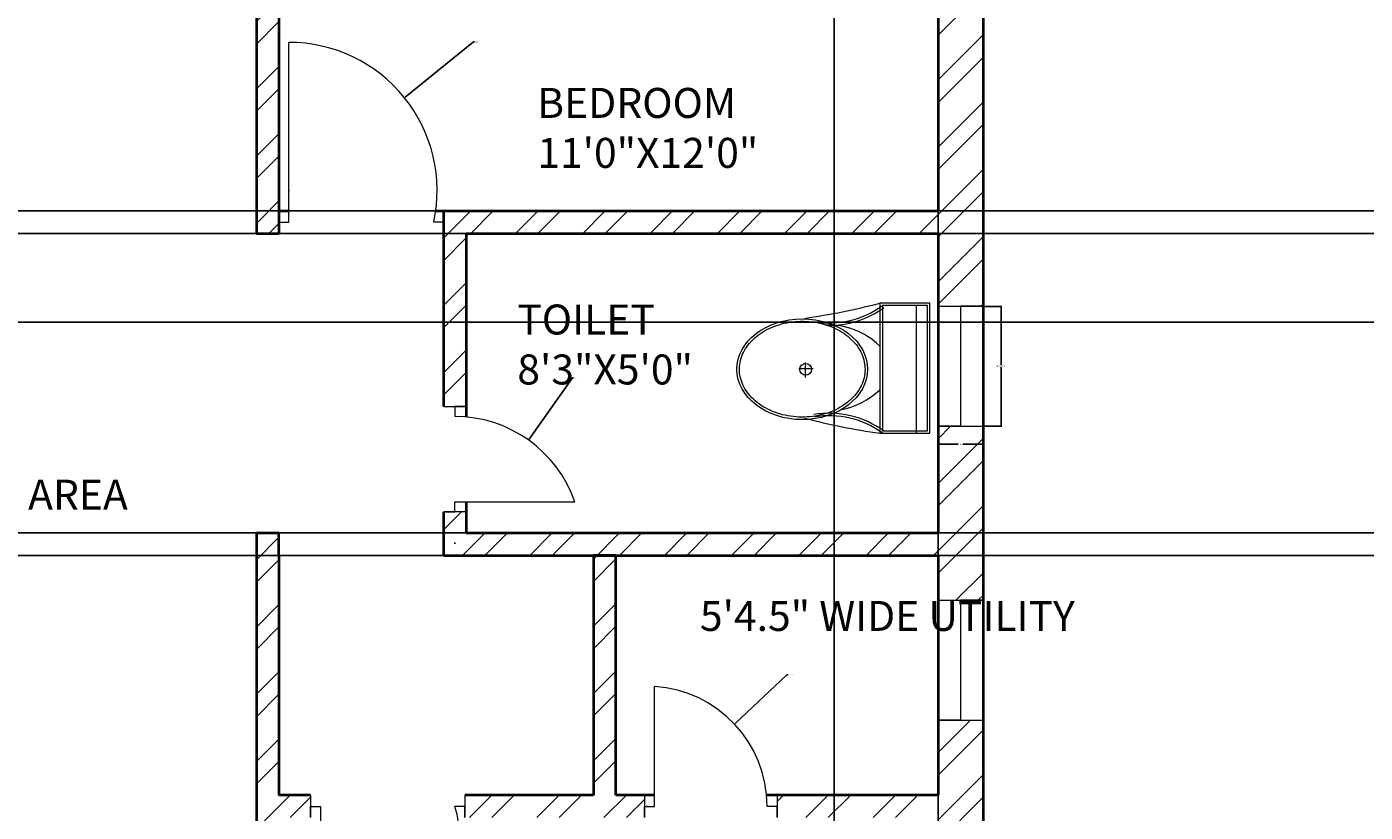
# Model space of a CAD drawing. Units: inches. Extents: x 1355 to 2746, y 1171 to 2751.
# Tile 12 of 24: x 1749 to 2017, y 1866 to 2023. Entities that reach past the tile are written whole.
import ezdxf

# ---------------------------------------------------------------- set-up
doc = ezdxf.new("R2010")
doc.units = ezdxf.units.IN
for name, color, linetype, lineweight in [('A-ANNO-DIMS', 2, 'Continuous', 18), ('A-AREA-IDEN', 7, 'Continuous', 18), ('A-DOOR', 3, 'Continuous', 20), ('A-FLOR-FIXT', 9, 'Continuous', 18), ('A-GLAZ', 4, 'Continuous', 18), ('A-WALL', 7, 'Continuous', 40), ('A-WALL-PATT', 252, 'Continuous', 13)]:
    doc.layers.add(name, color=color, linetype=linetype, lineweight=lineweight)
doc.styles.get("Standard").update_dxf_attribs({"font": 'arial.ttf'})
doc.dimstyles.get("Standard").update_dxf_attribs({"dimtxt": 0.18, "dimasz": 0.18, "dimexe": 0.18, "dimexo": 0.0625, "dimgap": 0.09, "dimtad": 0, "dimtih": 1, "dimtoh": 1, "dimdec": 4, "dimzin": 0, "dimdsep": 46, "dimtxsty": 'Standard', "dimcen": 0.09, "dimadec": 0, "dimazin": 0, "dimtfac": 1, "dimtdec": 4, "dimtofl": 0, "dimtmove": 0, "dimatfit": 3, "dimfxl": 1, "dimtolj": 1, "dimtzin": 0, "dimarcsym": 0})

# ---------------------------------------------------------------- blocks, each defined once
blk = doc.blocks.new('A$C31115884')
for p, q in [((283.1, 497.7), (223.4, 497.7)), ((257.5, 466.4), (257.5, 523.2)), ((0, 200), (0, 0)), ((520, 200), (0, 200)), ((10, 190), (10, 10)), ((510, 190), (10, 190)), ((510, 10), (510, 190)), ((520, 0), (520, 200)), ((510, 54.5), (0, 54.5)), ((10, 10), (510, 10)), ((0, 0), (520, 0))]:
    blk.add_line(p, q)
blk.add_circle((255.6, 496.4), 23.6)
for centre, radius, start, end in [((2777.7, -204.6), 2807, 165.4549, 171.7133), ((3237, 905), 2807, 188.2867, 194.5451), ((-294.5, 403.3), 364.7, 324.2091, 9.3499), ((-294.5, 403.3), 374.7, 324.2091, 9.3499), ((805.8, 403.3), 364.7, 170.6501, 215.7909), ((139.5, 406.2), 293.5, 315.8436, 2.6563), ((805.8, 403.3), 374.7, 179.2036, 215.7909), ((383.6, 406.2), 293.5, 190.2774, 224.1564)]:
    blk.add_arc(centre, radius, start, end)
blk.add_ellipse((256.2, 509.9), major_axis=(0, -260.7), ratio=0.772727)
blk.add_open_spline([(256.2, 259.2), (263.1, 259.2), (270, 259.7), (287.8, 262.3), (298.7, 265.1), (319.9, 273.1), (330.2, 278.4), (350.1, 291.1), (359.7, 298.7), (377.7, 315.9), (386.2, 325.5), (401.7, 346.6), (408.8, 358.1), (421.3, 382.5), (426.8, 395.5), (435.9, 422.4), (439.5, 436.4), (444.8, 465.1), (446.5, 479.7), (447.9, 509.2), (447.6, 524), (445, 553.3), (442.7, 567.8), (436.3, 596), (432.1, 609.7), (421.9, 636), (416, 648.6), (402.5, 672.1), (395, 683), (378.6, 703), (369.8, 712.1), (351.1, 728), (341.3, 734.8), (320.9, 746.2), (310.4, 750.7), (288.9, 757.3), (278, 759.4), (256, 761), (245, 760.6), (223.1, 757.2), (212.3, 754.3), (191.1, 746.1), (180.8, 740.7), (160.9, 727.8), (151.4, 720.1), (133.5, 702.7), (125.1, 693), (109.6, 671.7), (102.6, 660.2), (90.2, 635.7), (84.9, 622.7), (76, 595.6), (72.4, 581.6), (67.2, 552.9), (65.6, 538.2), (64.4, 508.8), (64.8, 494), (67.5, 464.7), (69.9, 450.2), (76.6, 422), (80.8, 408.3), (91.1, 382.2), (97.2, 369.7), (110.8, 346.3), (118.4, 335.4), (134.8, 315.6), (143.7, 306.7), (162.4, 290.9), (172.3, 284.2), (192.8, 273), (203.3, 268.6), (224.8, 262.2), (235.8, 260.2), (249.9, 259.3), (253, 259.2), (256.2, 259.2)], degree=3, knots=[0, 0, 0, 0, 0.110105, 0.110105, 0.285049, 0.285049, 0.459994, 0.459994, 0.634938, 0.634938, 0.809882, 0.809882, 0.984827, 0.984827, 1.159771, 1.159771, 1.334715, 1.334715, 1.50966, 1.50966, 1.684604, 1.684604, 1.859549, 1.859549, 2.034493, 2.034493, 2.209437, 2.209437, 2.384382, 2.384382, 2.559326, 2.559326, 2.73427, 2.73427, 2.909215, 2.909215, 3.084159, 3.084159, 3.259103, 3.259103, 3.434048, 3.434048, 3.608992, 3.608992, 3.783936, 3.783936, 3.958881, 3.958881, 4.133825, 4.133825, 4.30877, 4.30877, 4.483714, 4.483714, 4.658658, 4.658658, 4.833603, 4.833603, 5.008547, 5.008547, 5.183491, 5.183491, 5.358436, 5.358436, 5.53338, 5.53338, 5.708324, 5.708324, 5.883269, 5.883269, 6.058213, 6.058213, 6.233158, 6.233158, 6.283185, 6.283185, 6.283185, 6.283185])
blk = doc.blocks.new('WINDOW-PLAN-24')
for p, q in [((0, 24), (9, 24)), ((9, 24), (4.5, 24)), ((4.5, 24), (4.5, 0)), ((4.5, 0), (0, 0)), ((0, 0), (9, 0))]:
    blk.add_line(p, q)
blk = doc.blocks.new('WINDOW-PLAN-24-2')
for p, q in [((0, 24), (9, 24)), ((9, 24), (4.5, 24)), ((4.5, 24), (4.5, 0)), ((4.5, 0), (0, 0)), ((0, 0), (0, 0)), ((0, 0), (9, 0))]:
    blk.add_line(p, q)
blk = doc.blocks.new('DOOR-UTILITY-N')
for p, q in [((2, 2.25), (2, 26.25)), ((0, 4.5), (0, 0)), ((26.56, 4.5), (26.56, 0)), ((0, 0), (0, 2.25)), ((0, 2.25), (2, 2.25)), ((26.56, 2.25), (24.56, 2.25)), ((26.56, 0), (26.56, 2.25))]:
    blk.add_line(p, q)
blk.add_arc((0.51, 2.25), 24.05, 0, 86.4557)
blk = doc.blocks.new('DOOR-KITCHEN-N')
for p, q in [((0, 38.25), (0, 33.75)), ((30.9, 38.25), (30.9, 33.75)), ((0, 33.75), (0, 36)), ((0, 36), (2, 36)), ((2, 36), (2, 0)), ((30.9, 36), (28.9, 36)), ((30.9, 33.75), (30.9, 36))]:
    blk.add_line(p, q)
blk.add_arc((2, 28.05), 28.05, 270, 16.4594)
blk = doc.blocks.new('DOOR-BED-NE')
for p, q in [((2, 0), (2, 36)), ((33, 0.01), (31, 0.01)), ((0, 0), (2, 0))]:
    blk.add_line(p, q)
blk.add_arc((2, 6.32), 29.68, 347.7257, 90)
blk = doc.blocks.new('DOOR-WC-NE')
for p, q in [((0, 21.08), (4.5, 21.08)), ((4.5, 21.08), (2.25, 21.08)), ((2.25, 21.08), (2.25, 19.08)), ((4.5, 0), (0, 0)), ((0, 0), (2.25, 0)), ((2.25, 0), (2.25, 2)), ((2.25, 2), (26.25, 2))]:
    blk.add_line(p, q)
blk.add_arc((2.25, -6.32), 25.4, 19.1149, 90)
blk = doc.blocks.new('*D41')
at = {"layer": 'A-ANNO-DIMS', "color": 0, "lineweight": -2, "transparency": 16777216}
for p, q in [((1940.77, 1967.19), (1944.49, 1967.19)), ((1944.31, 1967.01), (1944.31, 1955.38)), ((1944.31, 1943.37), (1944.31, 1955.01)), ((1940.77, 1943.19), (1944.49, 1943.19))]:
    blk.add_line(p, q, dxfattribs=at)
at = {"layer": 'A-ANNO-DIMS', "color": 0, "transparency": 16777216}
for points in [[(1944.28, 1967.01), (1944.34, 1967.01), (1944.31, 1967.19)], [(1944.28, 1943.37), (1944.34, 1943.37), (1944.31, 1943.19)]]:
    blk.add_solid(points, dxfattribs=at)
at = {"layer": 'Defpoints', "color": 0, "transparency": 16777216}
for p in [(1940.71, 1967.19), (1944.31, 1967.19), (1940.71, 1943.19)]:
    blk.add_point(p, dxfattribs=at)
at = {"layer": 'A-ANNO-DIMS', "color": 0, "transparency": 16777216, "insert": (1944.31, 1955.19), "char_height": 0.18, "attachment_point": 5}
blk.add_mtext('\\A1;WINDOW 24 TYP.', dxfattribs=at)
blk = doc.blocks.new('*D42')
at = {"layer": 'A-ANNO-DIMS', "color": 0, "lineweight": -2, "transparency": 16777216}
for p, q in [((1931.71, 1943.13), (1931.71, 1939.41)), ((1940.71, 1943.13), (1940.71, 1939.41)), ((1931.89, 1939.59), (1935.75, 1939.59)), ((1940.53, 1939.59), (1936.67, 1939.59))]:
    blk.add_line(p, q, dxfattribs=at)
at = {"layer": 'A-ANNO-DIMS', "color": 0, "transparency": 16777216}
for points in [[(1931.89, 1939.62), (1931.89, 1939.56), (1931.71, 1939.59)], [(1940.53, 1939.62), (1940.53, 1939.56), (1940.71, 1939.59)]]:
    blk.add_solid(points, dxfattribs=at)
at = {"layer": 'Defpoints', "color": 0, "transparency": 16777216}
for p in [(1931.71, 1943.19), (1940.71, 1943.19), (1940.71, 1939.59)]:
    blk.add_point(p, dxfattribs=at)
at = {"layer": 'A-ANNO-DIMS', "color": 0, "transparency": 16777216, "insert": (1936.21, 1939.59), "char_height": 0.18, "attachment_point": 5}
blk.add_mtext('\\A1;9 TYP.', dxfattribs=at)
blk = doc.blocks.new('*D103')
at = {"layer": 'A-ANNO-DIMS', "color": 0, "lineweight": -2, "transparency": 16777216}
for p, q in [((2089.33, 1917.3), (1407.53, 1917.3)), ((1407.71, 1917.12), (1407.71, 1840.98)), ((1407.71, 1764.48), (1407.71, 1840.62)), ((2089.33, 1764.3), (1407.53, 1764.3))]:
    blk.add_line(p, q, dxfattribs=at)
at = {"layer": 'A-ANNO-DIMS', "color": 0, "transparency": 16777216}
for points in [[(1407.68, 1917.12), (1407.74, 1917.12), (1407.71, 1917.3)], [(1407.68, 1764.48), (1407.74, 1764.48), (1407.71, 1764.3)]]:
    blk.add_solid(points, dxfattribs=at)
at = {"layer": 'Defpoints', "color": 0, "transparency": 16777216}
for p in [(1407.71, 1917.3), (2089.39, 1917.3), (2089.39, 1764.3)]:
    blk.add_point(p, dxfattribs=at)
at = {"layer": 'A-ANNO-DIMS', "color": 0, "transparency": 16777216, "insert": (1407.71, 1840.8), "char_height": 0.18, "attachment_point": 5}
blk.add_mtext('\\A1;153', dxfattribs=at)
blk = doc.blocks.new('*D104')
at = {"layer": 'A-ANNO-DIMS', "color": 0, "lineweight": -2, "transparency": 16777216}
for p, q in [((2089.33, 1986.3), (1407.53, 1986.3)), ((1407.71, 1986.12), (1407.71, 1951.98)), ((1407.71, 1917.48), (1407.71, 1951.62)), ((2089.33, 1917.3), (1407.53, 1917.3))]:
    blk.add_line(p, q, dxfattribs=at)
at = {"layer": 'A-ANNO-DIMS', "color": 0, "transparency": 16777216}
for points in [[(1407.68, 1986.12), (1407.74, 1986.12), (1407.71, 1986.3)], [(1407.68, 1917.48), (1407.74, 1917.48), (1407.71, 1917.3)]]:
    blk.add_solid(points, dxfattribs=at)
at = {"layer": 'Defpoints', "color": 0, "transparency": 16777216}
for p in [(1407.71, 1986.3), (2089.39, 1986.3), (2089.39, 1917.3)]:
    blk.add_point(p, dxfattribs=at)
at = {"layer": 'A-ANNO-DIMS', "color": 0, "transparency": 16777216, "insert": (1407.71, 1951.8), "char_height": 0.18, "attachment_point": 5}
blk.add_mtext('\\A1;69', dxfattribs=at)
blk = doc.blocks.new('*D105')
at = {"layer": 'A-ANNO-DIMS', "color": 0, "lineweight": -2, "transparency": 16777216}
for p, q in [((2080.33, 2139.3), (1407.53, 2139.3)), ((1407.71, 2139.12), (1407.71, 2062.98)), ((1407.71, 1986.48), (1407.71, 2062.62)), ((2089.33, 1986.3), (1407.53, 1986.3))]:
    blk.add_line(p, q, dxfattribs=at)
at = {"layer": 'A-ANNO-DIMS', "color": 0, "transparency": 16777216}
for points in [[(1407.68, 2139.12), (1407.74, 2139.12), (1407.71, 2139.3)], [(1407.68, 1986.48), (1407.74, 1986.48), (1407.71, 1986.3)]]:
    blk.add_solid(points, dxfattribs=at)
at = {"layer": 'Defpoints', "color": 0, "transparency": 16777216}
for p in [(1407.71, 2139.3), (2080.39, 2139.3), (2089.39, 1986.3)]:
    blk.add_point(p, dxfattribs=at)
at = {"layer": 'A-ANNO-DIMS', "color": 0, "transparency": 16777216, "insert": (1407.71, 2062.8), "char_height": 0.18, "attachment_point": 5}
blk.add_mtext('\\A1;153', dxfattribs=at)
blk = doc.blocks.new('*D136')
at = {"layer": 'A-ANNO-DIMS', "color": 0, "lineweight": -2, "transparency": 16777216}
for p, q in [((1618.27, 1981.8), (2648.07, 1981.8)), ((2647.89, 1981.62), (2647.89, 1951.98)), ((2647.89, 1921.98), (2647.89, 1951.62)), ((1618.27, 1921.8), (2648.07, 1921.8))]:
    blk.add_line(p, q, dxfattribs=at)
at = {"layer": 'A-ANNO-DIMS', "color": 0, "transparency": 16777216}
for points in [[(2647.86, 1981.62), (2647.92, 1981.62), (2647.89, 1981.8)], [(2647.86, 1921.98), (2647.92, 1921.98), (2647.89, 1921.8)]]:
    blk.add_solid(points, dxfattribs=at)
at = {"layer": 'Defpoints', "color": 0, "transparency": 16777216}
for p in [(1618.21, 1981.8), (2647.89, 1981.8), (1618.21, 1921.8)]:
    blk.add_point(p, dxfattribs=at)
at = {"layer": 'A-ANNO-DIMS', "color": 0, "transparency": 16777216, "insert": (2647.89, 1951.8), "char_height": 0.18, "attachment_point": 5}
blk.add_mtext('\\A1;60', dxfattribs=at)
blk = doc.blocks.new('*D139')
at = {"layer": 'A-ANNO-DIMS', "color": 0, "lineweight": -2, "transparency": 16777216}
for p, q in [((1523.77, 1981.8), (2648.07, 1981.8)), ((2647.89, 1981.62), (2647.89, 1973.09)), ((2647.89, 1964.19), (2647.89, 1972.72)), ((1548.66, 1964.01), (2648.07, 1964.01))]:
    blk.add_line(p, q, dxfattribs=at)
at = {"layer": 'A-ANNO-DIMS', "color": 0, "transparency": 16777216}
for points in [[(2647.86, 1981.62), (2647.92, 1981.62), (2647.89, 1981.8)], [(2647.86, 1964.19), (2647.92, 1964.19), (2647.89, 1964.01)]]:
    blk.add_solid(points, dxfattribs=at)
at = {"layer": 'Defpoints', "color": 0, "transparency": 16777216}
for p in [(1523.71, 1981.8), (1548.6, 1964.01), (2647.89, 1964.01)]:
    blk.add_point(p, dxfattribs=at)
at = {"layer": 'A-ANNO-DIMS', "color": 0, "transparency": 16777216, "insert": (2647.89, 1972.9), "char_height": 0.18, "attachment_point": 5}
blk.add_mtext('\\A1;17.795', dxfattribs=at)
blk = doc.blocks.new('*D145')
at = {"layer": 'A-ANNO-DIMS', "color": 0, "lineweight": -2, "transparency": 16777216}
for p, q in [((1910.88, 1399.86), (1910.88, 2716.58)), ((1911.06, 2716.4), (1920.83, 2716.4)), ((1931.53, 2716.4), (1921.76, 2716.4)), ((1931.71, 1399.86), (1931.71, 2716.58))]:
    blk.add_line(p, q, dxfattribs=at)
at = {"layer": 'A-ANNO-DIMS', "color": 0, "transparency": 16777216}
for points in [[(1911.06, 2716.43), (1911.06, 2716.37), (1910.88, 2716.4)], [(1931.53, 2716.43), (1931.53, 2716.37), (1931.71, 2716.4)]]:
    blk.add_solid(points, dxfattribs=at)
at = {"layer": 'Defpoints', "color": 0, "transparency": 16777216}
for p in [(1931.71, 2716.4), (1910.88, 1399.8), (1931.71, 1399.8)]:
    blk.add_point(p, dxfattribs=at)
at = {"layer": 'A-ANNO-DIMS', "color": 0, "transparency": 16777216, "insert": (1921.3, 2716.4), "char_height": 0.18, "attachment_point": 5}
blk.add_mtext('\\A1;20.824', dxfattribs=at)
blk = doc.blocks.new('*D156')
at = {"layer": 'A-ANNO-DIMS', "color": 0, "lineweight": -2, "transparency": 16777216}
for p, q in [((1838.68, 2020.17), (1824.96, 2009.11)), ((1838.86, 2020.17), (1838.68, 2020.17)), ((1801.62, 1990.37), (1801.8, 1990.37)), ((1801.71, 1990.28), (1801.71, 1990.46))]:
    blk.add_line(p, q, dxfattribs=at)
at = {"layer": 'A-ANNO-DIMS', "color": 0, "transparency": 16777216}
blk.add_solid([(1824.94, 2009.13), (1824.98, 2009.08), (1824.82, 2009)], dxfattribs=at)
at = {"layer": 'Defpoints', "color": 0, "transparency": 16777216}
for p in [(1824.82, 2009), (1801.71, 1990.37)]:
    blk.add_point(p, dxfattribs=at)
at = {"layer": 'A-ANNO-DIMS', "color": 0, "transparency": 16777216, "insert": (1839.34, 2020.17), "char_height": 0.18, "attachment_point": 5}
blk.add_mtext('\\A1;R29.68', dxfattribs=at)
blk = doc.blocks.new('*D160')
at = {"layer": 'A-ANNO-DIMS', "color": 0, "lineweight": -2, "transparency": 16777216}
for p, q in [((1858.53, 1952.84), (1849.79, 1940.57)), ((1858.71, 1952.84), (1858.53, 1952.84)), ((1834.87, 1919.73), (1835.05, 1919.73)), ((1834.96, 1919.64), (1834.96, 1919.82))]:
    blk.add_line(p, q, dxfattribs=at)
at = {"layer": 'A-ANNO-DIMS', "color": 0, "transparency": 16777216}
blk.add_solid([(1849.77, 1940.59), (1849.82, 1940.56), (1849.69, 1940.43)], dxfattribs=at)
at = {"layer": 'Defpoints', "color": 0, "transparency": 16777216}
for p in [(1849.69, 1940.43), (1834.96, 1919.73)]:
    blk.add_point(p, dxfattribs=at)
at = {"layer": 'A-ANNO-DIMS', "color": 0, "transparency": 16777216, "insert": (1859.12, 1952.84), "char_height": 0.18, "attachment_point": 5}
blk.add_mtext('\\A1;R25.4', dxfattribs=at)
blk = doc.blocks.new('*D162')
at = {"layer": 'A-ANNO-DIMS', "color": 0, "lineweight": -2, "transparency": 16777216}
for p, q in [((1901.45, 1893.4), (1891.06, 1883.64)), ((1901.63, 1893.4), (1901.45, 1893.4)), ((1873.32, 1867.05), (1873.5, 1867.05)), ((1873.41, 1866.96), (1873.41, 1867.14))]:
    blk.add_line(p, q, dxfattribs=at)
at = {"layer": 'A-ANNO-DIMS', "color": 0, "transparency": 16777216}
blk.add_solid([(1891.04, 1883.67), (1891.08, 1883.62), (1890.93, 1883.52)], dxfattribs=at)
at = {"layer": 'Defpoints', "color": 0, "transparency": 16777216}
for p in [(1890.93, 1883.52), (1873.41, 1867.05)]:
    blk.add_point(p, dxfattribs=at)
at = {"layer": 'A-ANNO-DIMS', "color": 0, "transparency": 16777216, "insert": (1902.18, 1893.4), "char_height": 0.18, "attachment_point": 5}
blk.add_mtext('\\A1;R24.046', dxfattribs=at)

msp = doc.modelspace()

# ---------------------------------------------------------------- hatches: boundary and pattern name
at = {"layer": 'A-WALL-PATT'}
h = msp.add_hatch(dxfattribs=at)
h.set_pattern_fill('ANSI32', color=256)
h.paths.add_polyline_path([(1660.2083, 2139.3018), (1614.5977, 2139.3018), (1614.5977, 2130.3018), (1655.7083, 2130.3018), (1655.7083, 1981.8018), (1660.2083, 1981.8018), (1660.2083, 2090.7225), (1692.5832, 2090.7225), (1692.5832, 2095.2225), (1660.2083, 2095.2225)])
h.paths.add_polyline_path([(1523.7083, 2130.3018), (1554.5977, 2130.3018), (1554.5977, 2134.8018), (1554.5977, 2139.3018), (1514.7083, 2139.3018), (1514.7083, 2071.8385), (1523.7083, 2071.8385)])
h.paths.add_polyline_path([(1940.7083, 2139.3018), (1883.7928, 2139.3018), (1883.7928, 2130.3018), (1931.7083, 2130.3018), (1931.7083, 2098.3333), (1940.7083, 2098.3333)])
h.paths.add_polyline_path([(1799.7083, 2130.3018), (1823.7928, 2130.3018), (1823.7928, 2134.8018), (1823.7928, 2139.3018), (1795.2083, 2139.3018), (1795.2083, 2130.3018), (1795.2083, 2095.2225), (1759.2134, 2095.2225), (1759.2134, 2090.7225), (1795.2083, 2090.7225), (1795.2083, 1981.8018), (1799.7083, 1981.8018), (1799.7083, 1986.3018)])
h.paths.add_polyline_path([(1940.7083, 2038.3333), (1931.7083, 2038.3333), (1931.7083, 1986.3018), (1832.7083, 1986.3018), (1832.7083, 1947.1338), (1837.2083, 1947.1338), (1837.2083, 1981.8018), (1931.7083, 1981.8018), (1931.7083, 1967.1939), (1940.7083, 1967.1939)])
h.paths.add_polyline_path([(1940.7083, 1943.1939), (1931.7083, 1943.1939), (1931.7083, 1921.8018), (1837.2083, 1921.8018), (1837.2083, 1926.0511), (1832.7083, 1926.0511), (1832.7083, 1917.3018), (1931.7083, 1917.3018), (1931.7083, 1908.3321), (1940.7083, 1908.3321)])
h.paths.add_polyline_path([(1940.7083, 1884.3321), (1931.7083, 1884.3321), (1931.7083, 1869.3018), (1899.4583, 1869.3018), (1899.4583, 1864.8018), (1931.7083, 1864.8018), (1931.7083, 1773.3018), (1786.5143, 1773.3018), (1786.5143, 1764.3018), (1844.7083, 1764.3018), (1844.7083, 1748.9343), (1853.7083, 1748.9343), (1853.7083, 1764.3018), (1931.7083, 1764.3018), (1931.7083, 1652.9424), (1940.7083, 1652.9424)])
h.paths.add_polyline_path([(1799.7083, 1864.8018), (1806.0522, 1864.8018), (1806.0522, 1867.0518), (1806.0522, 1869.3018), (1799.7083, 1869.3018), (1799.7083, 1917.3018), (1799.7083, 1921.8018), (1795.2083, 1921.8018), (1795.2083, 1773.3018), (1799.7083, 1773.3018)])
h.paths.add_polyline_path([(1872.8988, 1867.0518), (1872.8988, 1869.3018), (1867.2083, 1869.3018), (1867.2083, 1917.3018), (1862.7083, 1917.3018), (1862.7083, 1869.3018), (1836.9546, 1869.3018), (1836.9546, 1864.8018), (1862.7083, 1864.8018), (1872.8988, 1864.8018)])
h.paths.add_polyline_path([(1749.2197, 1773.3018), (1655.7083, 1773.3018), (1523.7083, 1773.3018), (1523.7083, 1828.4963), (1514.7083, 1828.4963), (1514.7083, 1753.9033), (1519.2083, 1753.9033), (1523.7083, 1753.9033), (1523.7083, 1764.3018), (1655.7083, 1764.3018), (1749.2197, 1764.3018), (1749.2197, 1768.8018)])
h.paths.add_polyline_path([(1660.2083, 1921.8018), (1655.7083, 1921.8018), (1655.7083, 1917.3018), (1655.7083, 1773.3018), (1660.2083, 1773.3018)])
h.paths.add_polyline_path([(1523.7083, 2011.8385), (1514.7083, 2011.8385), (1514.7083, 1973.114), (1519.2083, 1973.114), (1523.7083, 1973.114), (1523.7083, 1976.8227), (1523.7083, 1981.8018), (1618.2083, 1981.8018), (1618.2083, 1921.8018), (1553.707, 1921.8018), (1553.707, 1917.3018), (1622.7083, 1917.3018), (1622.7083, 1919.5518), (1622.7083, 1921.8018), (1622.7083, 1986.3018), (1523.7083, 1986.3018)])
h.paths.add_polyline_path([(1529.6686, 1919.5518), (1529.6686, 1921.8018), (1523.7083, 1921.8018), (1523.7083, 1949.114), (1514.7083, 1949.114), (1514.7083, 1888.4963), (1523.7083, 1888.4963), (1523.7083, 1917.3018), (1529.6686, 1917.3018)])
h.paths.add_polyline_path([(1538.9419, 1775.643), (1585.5504, 1775.643), (1585.5504, 1798.0318), (1538.9419, 1798.0318)], flags=25)
h.paths.add_polyline_path([(1696.7097, 1497.3356), (1769.5651, 1497.3356), (1769.5651, 1523.4559), (1696.7097, 1523.4559)], flags=9)
h.paths.add_polyline_path([(1629.1643, 1230.5133), (1877.0879, 1230.5133), (1877.0879, 1267.606), (1629.1643, 1267.606)], flags=9)
h.paths.add_polyline_path([(2533.4462, 2215.4033), (2579.9292, 2215.4033), (2579.9292, 2231.889), (2533.4462, 2231.889)], flags=9)
h.paths.add_polyline_path([(2540.822, 2515.6945), (2594.2245, 2515.6945), (2594.2245, 2545.5463), (2540.822, 2545.5463)], flags=9)
h.paths.add_polyline_path([(2535.9857, 2588.2819), (2582.4687, 2588.2819), (2582.4687, 2604.7675), (2535.9857, 2604.7675)], flags=9)
h.paths.add_polyline_path([(2537.1627, 2617.1172), (2649.1245, 2617.1172), (2649.1245, 2633.6029), (2537.1627, 2633.6029)], flags=9)
h.paths.add_polyline_path([(2218.0051, 2168.228), (2363.9573, 2168.228), (2363.9573, 2205.3208), (2218.0051, 2205.3208)], flags=9)
h.paths.add_polyline_path([(1650.2156, 2165.3631), (1800.3547, 2165.3631), (1800.3547, 2202.4559), (1650.2156, 2202.4559)], flags=9)
h.paths.add_polyline_path([(2553.9592, 1610.7663), (2588.4203, 1610.7663), (2588.4203, 1660.2233), (2553.9592, 1660.2233)], flags=9)
h.paths.add_polyline_path([(1549.0868, 1648.2033), (1595.6952, 1648.2033), (1595.6952, 1670.5921), (1549.0868, 1670.5921)], flags=9)
h.paths.add_polyline_path([(1546.9525, 1502.0931), (1583.3413, 1502.0931), (1583.3413, 1524.4819), (1546.9525, 1524.4819)], flags=9)
h.paths.add_polyline_path([(1540.7704, 1433.4431), (1587.3788, 1433.4431), (1587.3788, 1455.8319), (1540.7704, 1455.8319)], flags=9)
h.paths.add_polyline_path([(1683.6524, 1321.5269), (1760.6169, 1321.5269), (1760.6169, 1333.8911), (1683.6524, 1333.8911)], flags=9)
h.paths.add_polyline_path([(1832.0485, 1356.0874), (1873.0989, 1356.0874), (1873.0989, 1378.4762), (1832.0485, 1378.4762)], flags=9)
h.paths.add_polyline_path([(1877.9694, 1431.2138), (1926.3827, 1431.2138), (1926.3827, 1453.578), (1877.9694, 1453.578)], flags=9)
h.paths.add_polyline_path([(1847.3106, 1499.8371), (1883.6994, 1499.8371), (1883.6994, 1522.2259), (1847.3106, 1522.2259)], flags=9)
h.paths.add_polyline_path([(1813.7015, 1640.7287), (1860.3099, 1640.7287), (1860.3099, 1663.1175), (1813.7015, 1663.1175)], flags=9)
h.paths.add_polyline_path([(1876.2576, 1710.2471), (1912.9452, 1710.2471), (1912.9452, 1732.6359), (1876.2576, 1732.6359)], flags=25)
h.paths.add_polyline_path([(1695.9163, 1715.3064), (1736.9668, 1715.3064), (1736.9668, 1737.6952), (1695.9163, 1737.6952)], flags=9)
h.paths.add_polyline_path([(1881.8583, 1888.9094), (1930.2717, 1888.9094), (1930.2717, 1911.2737), (1881.8583, 1911.2737)], flags=9)
h.paths.add_polyline_path([(1823.9298, 1798.6431), (1864.9803, 1798.6431), (1864.9803, 1821.0319), (1823.9298, 1821.0319)], flags=25)
h.paths.add_polyline_path([(1845.6062, 1948.1408), (1881.995, 1948.1408), (1881.995, 1970.5296), (1845.6062, 1970.5296)], flags=25)
h.paths.add_polyline_path([(1849.027, 1991.5151), (1895.6355, 1991.5151), (1895.6355, 2013.9039), (1849.027, 2013.9039)], flags=25)
h.paths.add_polyline_path([(1684.9725, 2113.8416), (1764.2658, 2113.8416), (1764.2658, 2126.2058), (1684.9725, 2126.2058)], flags=9)
h.paths.add_polyline_path([(1688.6193, 1913.0676), (1776.2005, 1913.0676), (1776.2005, 1935.4564), (1688.6193, 1935.4564)], flags=9)
h.paths.add_polyline_path([(1571.4689, 1930.9816), (1607.8577, 1930.9816), (1607.8577, 1953.3704), (1571.4689, 1953.3704)], flags=25)
h.paths.add_polyline_path([(1535.3581, 1998.3125), (1581.9665, 1998.3125), (1581.9665, 2020.7014), (1535.3581, 2020.7014)], flags=9)
h = msp.add_hatch(dxfattribs=at)
h.set_pattern_fill('ANSI32', color=256)
h.paths.add_polyline_path([(1749.2197, 1686.3018), (1732.6892, 1686.3018), (1523.7083, 1686.3018), (1523.7083, 1705.9033), (1514.7083, 1705.9033), (1514.7083, 1647.8732), (1519.2083, 1647.8732), (1523.7083, 1647.8732), (1523.7083, 1677.3018), (1655.7083, 1677.3018), (1655.7083, 1528.8018), (1660.2083, 1528.8018), (1660.2083, 1677.3018), (1732.6892, 1677.3018), (1749.2197, 1677.3018)])
h.paths.add_polyline_path([(1931.7083, 1686.3018), (1853.7083, 1686.3018), (1853.7083, 1703.5696), (1844.7083, 1703.5696), (1844.7083, 1686.3018), (1788.0274, 1686.3018), (1788.0274, 1677.3018), (1795.2083, 1677.3018), (1795.2083, 1528.8018), (1799.7083, 1528.8018), (1799.7083, 1677.3018), (1844.7083, 1677.3018), (1931.7083, 1677.3018)])
h.paths.add_polyline_path([(1931.7083, 1533.3018), (1844.7083, 1533.3018), (1832.7083, 1533.3018), (1832.7083, 1531.0518), (1832.7083, 1528.8018), (1832.7083, 1495.7519), (1837.2083, 1495.7519), (1837.2083, 1528.8018), (1931.7083, 1528.8018)])
h.paths.add_polyline_path([(1940.7083, 1592.9424), (1931.7083, 1592.9424), (1931.7083, 1506.7845), (1940.7083, 1506.7845)])
h.paths.add_polyline_path([(1940.7083, 1482.7845), (1936.2083, 1482.7845), (1931.7083, 1482.7845), (1931.7083, 1320.3018), (1880.7083, 1320.3018), (1880.7083, 1311.3018), (1940.7083, 1311.3018)])
h.paths.add_polyline_path([(1931.7083, 1468.8018), (1844.7083, 1468.8018), (1837.2083, 1468.8018), (1837.2083, 1474.34), (1832.7083, 1474.34), (1832.7083, 1468.8018), (1832.7083, 1464.3018), (1844.7083, 1464.3018), (1931.7083, 1464.3018)])
h.paths.add_polyline_path([(1863.8571, 1464.3018), (1859.3571, 1464.3018), (1859.3571, 1404.1662), (1838.1542, 1404.1662), (1838.1542, 1399.8018), (1869.4185, 1399.8018), (1869.4185, 1402.0518), (1869.4185, 1404.3018), (1863.8571, 1404.3018)])
h.paths.add_polyline_path([(1799.7083, 1399.6662), (1805.4082, 1399.6662), (1805.4082, 1401.9162), (1805.4082, 1404.1662), (1799.7083, 1404.1662), (1799.7083, 1464.3018), (1799.7083, 1468.8018), (1795.2083, 1468.8018), (1795.2083, 1356.2098), (1761.2597, 1356.2098), (1761.2597, 1351.7098), (1795.2083, 1351.7098), (1795.2083, 1320.3018), (1795.2083, 1311.3018), (1844.7083, 1311.3018), (1844.7083, 1315.8018), (1844.7083, 1320.3018), (1799.7083, 1320.3018)])
h.paths.add_polyline_path([(1692.9218, 1356.2098), (1660.2083, 1356.2098), (1660.2083, 1430.786), (1657.9583, 1430.786), (1655.7083, 1430.786), (1655.7083, 1320.3018), (1611.934, 1320.3018), (1611.934, 1311.3018), (1660.2083, 1311.3018), (1660.2083, 1351.7098), (1692.9218, 1351.7098)])
h.paths.add_polyline_path([(1523.7083, 1372.653), (1514.7083, 1372.653), (1514.7083, 1311.3018), (1551.934, 1311.3018), (1551.934, 1315.8018), (1551.934, 1320.3018), (1523.7083, 1320.3018)])
h.paths.add_polyline_path([(1523.7083, 1490.9023), (1514.7083, 1490.9023), (1514.7083, 1432.653), (1519.2083, 1432.653), (1523.7083, 1432.653)])
h.paths.add_polyline_path([(1660.2083, 1468.8018), (1622.7083, 1468.8018), (1622.7083, 1473.1566), (1618.2083, 1473.1566), (1618.2083, 1468.8018), (1523.7083, 1468.8018), (1523.7083, 1464.3018), (1655.7083, 1464.3018), (1655.7083, 1460.5634), (1660.2083, 1460.5634)])
h.paths.add_polyline_path([(1523.7083, 1587.8732), (1514.7083, 1587.8732), (1514.7083, 1514.9023), (1519.2083, 1514.9023), (1523.7083, 1514.9023)])
h.paths.add_polyline_path([(1622.7083, 1533.3018), (1523.7083, 1533.3018), (1523.7083, 1528.8018), (1618.2083, 1528.8018), (1618.2083, 1494.4205), (1622.7083, 1494.4205), (1622.7083, 1528.8018)])
h.paths.add_polyline_path([(1696.7097, 1497.3356), (1769.5651, 1497.3356), (1769.5651, 1523.4559), (1696.7097, 1523.4559)], flags=9)
h.paths.add_polyline_path([(1629.1643, 1230.5133), (1877.0879, 1230.5133), (1877.0879, 1267.606), (1629.1643, 1267.606)], flags=9)
h.paths.add_polyline_path([(2533.4462, 2215.4033), (2579.9292, 2215.4033), (2579.9292, 2231.889), (2533.4462, 2231.889)], flags=9)
h.paths.add_polyline_path([(2540.822, 2515.6945), (2594.2245, 2515.6945), (2594.2245, 2545.5463), (2540.822, 2545.5463)], flags=9)
h.paths.add_polyline_path([(2535.9857, 2588.2819), (2582.4687, 2588.2819), (2582.4687, 2604.7675), (2535.9857, 2604.7675)], flags=9)
h.paths.add_polyline_path([(2537.1627, 2617.1172), (2649.1245, 2617.1172), (2649.1245, 2633.6029), (2537.1627, 2633.6029)], flags=9)
h.paths.add_polyline_path([(2218.0051, 2168.228), (2363.9573, 2168.228), (2363.9573, 2205.3208), (2218.0051, 2205.3208)], flags=9)
h.paths.add_polyline_path([(1650.2156, 2165.3631), (1800.3547, 2165.3631), (1800.3547, 2202.4559), (1650.2156, 2202.4559)], flags=9)
h.paths.add_polyline_path([(2553.9592, 1610.7663), (2588.4203, 1610.7663), (2588.4203, 1660.2233), (2553.9592, 1660.2233)], flags=9)
h.paths.add_polyline_path([(1549.0868, 1648.2033), (1595.6952, 1648.2033), (1595.6952, 1670.5921), (1549.0868, 1670.5921)], flags=25)
h.paths.add_polyline_path([(1546.9525, 1502.0931), (1583.3413, 1502.0931), (1583.3413, 1524.4819), (1546.9525, 1524.4819)], flags=25)
h.paths.add_polyline_path([(1540.7704, 1433.4431), (1587.3788, 1433.4431), (1587.3788, 1455.8319), (1540.7704, 1455.8319)], flags=9)
h.paths.add_polyline_path([(1683.6524, 1321.5269), (1760.6169, 1321.5269), (1760.6169, 1333.8911), (1683.6524, 1333.8911)], flags=9)
h.paths.add_polyline_path([(1832.0485, 1356.0874), (1873.0989, 1356.0874), (1873.0989, 1378.4762), (1832.0485, 1378.4762)], flags=9)
h.paths.add_polyline_path([(1877.9694, 1431.2138), (1926.3827, 1431.2138), (1926.3827, 1453.578), (1877.9694, 1453.578)], flags=9)
h.paths.add_polyline_path([(1847.3106, 1499.8371), (1883.6994, 1499.8371), (1883.6994, 1522.2259), (1847.3106, 1522.2259)], flags=25)
h.paths.add_polyline_path([(1813.7015, 1640.7287), (1860.3099, 1640.7287), (1860.3099, 1663.1175), (1813.7015, 1663.1175)], flags=25)
h.paths.add_polyline_path([(1876.2576, 1710.2471), (1912.9452, 1710.2471), (1912.9452, 1732.6359), (1876.2576, 1732.6359)], flags=9)
h.paths.add_polyline_path([(1695.9163, 1715.3064), (1736.9668, 1715.3064), (1736.9668, 1737.6952), (1695.9163, 1737.6952)], flags=9)
h.paths.add_polyline_path([(1881.8583, 1888.9094), (1930.2717, 1888.9094), (1930.2717, 1911.2737), (1881.8583, 1911.2737)], flags=9)
h.paths.add_polyline_path([(1823.9298, 1798.6431), (1864.9803, 1798.6431), (1864.9803, 1821.0319), (1823.9298, 1821.0319)], flags=9)
h.paths.add_polyline_path([(1845.6062, 1948.1408), (1881.995, 1948.1408), (1881.995, 1970.5296), (1845.6062, 1970.5296)], flags=9)
h.paths.add_polyline_path([(1849.027, 1991.5151), (1895.6355, 1991.5151), (1895.6355, 2013.9039), (1849.027, 2013.9039)], flags=9)
h.paths.add_polyline_path([(1684.9725, 2113.8416), (1764.2658, 2113.8416), (1764.2658, 2126.2058), (1684.9725, 2126.2058)], flags=9)
h.paths.add_polyline_path([(1688.6193, 1913.0676), (1776.2005, 1913.0676), (1776.2005, 1935.4564), (1688.6193, 1935.4564)], flags=9)
h.paths.add_polyline_path([(1538.9419, 1775.643), (1585.5504, 1775.643), (1585.5504, 1798.0318), (1538.9419, 1798.0318)], flags=9)
h.paths.add_polyline_path([(1571.4689, 1930.9816), (1607.8577, 1930.9816), (1607.8577, 1953.3704), (1571.4689, 1953.3704)], flags=9)
h.paths.add_polyline_path([(1535.3581, 1998.3125), (1581.9665, 1998.3125), (1581.9665, 2020.7014), (1535.3581, 2020.7014)], flags=9)

# ---------------------------------------------------------------- linework, layer by layer
at = {"layer": 'A-WALL'}
for p, q in [((1940.7083, 2139.3018), (1940.7083, 1311.3018)), ((1799.7083, 2130.3018), (1799.7083, 1986.3018)), ((1931.7083, 2130.3018), (1931.7083, 1986.3018)), ((1795.2083, 2090.7225), (1795.2083, 1981.8018)), ((1799.7083, 1986.3018), (1801.7083, 1986.3018)), ((1799.7083, 1986.3018), (1799.7083, 1981.8018)), ((1831.1061, 1986.3018), (1931.7083, 1986.3018)), ((1832.7083, 1986.3018), (1837.2083, 1986.3018)), ((1832.7083, 1947.1338), (1832.7083, 1986.3018)), ((1795.2083, 1981.8018), (1799.7083, 1981.8018)), ((1837.2083, 1981.8018), (1837.2083, 1945.034)), ((1837.2083, 1981.8018), (1931.7083, 1981.8018)), ((1931.7083, 1981.8018), (1931.7083, 1921.8018)), ((1837.2083, 1928.0511), (1837.2083, 1921.8018)), ((1832.7083, 1917.3018), (1832.7083, 1926.0511)), ((1795.2083, 1921.8018), (1795.2083, 1773.3018)), ((1795.2083, 1921.8018), (1799.7083, 1921.8018)), ((1799.7083, 1917.3018), (1799.7083, 1921.8018)), ((1837.2083, 1921.8018), (1931.7083, 1921.8018)), ((1799.7083, 1917.3018), (1799.7083, 1869.3018)), ((1832.7083, 1917.3018), (1931.7083, 1917.3018)), ((1867.2083, 1917.3018), (1862.7083, 1917.3018)), ((1862.7083, 1917.3018), (1862.7083, 1869.3018)), ((1867.2083, 1869.3018), (1867.2083, 1917.3018)), ((1931.7083, 1917.3018), (1931.7083, 1869.3018)), ((1931.7083, 1917.3018), (1931.7083, 1869.3018)), ((1806.0522, 1869.3018), (1799.7083, 1869.3018)), ((1862.7083, 1869.3018), (1836.9546, 1869.3018)), ((1874.8988, 1869.3018), (1867.2083, 1869.3018)), ((1931.7083, 1869.3018), (1897.3528, 1869.3018))]:
    msp.add_line(p, q, dxfattribs=at)

# ---------------------------------------------------------------- block references
at = {"layer": 'A-DOOR'}
for name, p in [('DOOR-BED-NE', (1799.708, 1984.052)), ('DOOR-WC-NE', (1832.708, 1926.051)), ('DOOR-UTILITY-N', (1872.899, 1864.802)), ('DOOR-KITCHEN-N', (1806.052, 1831.052))]:
    msp.add_blockref(name, p, dxfattribs=at)
at = {"layer": 'A-FLOR-FIXT', "xscale": 0.0501345278177945, "yscale": 0.0501345278177945, "zscale": 0.0501345278177945, "rotation": 89.99999999999999}
msp.add_blockref('A$C31115884', (1930.0724, 1941.7586), dxfattribs=at)
at = {"layer": 'A-GLAZ'}
for name, p in [('WINDOW-PLAN-24', (1931.708, 1943.194)), ('WINDOW-PLAN-24-2', (1931.708, 1884.332))]:
    msp.add_blockref(name, p, dxfattribs=at)

# ---------------------------------------------------------------- texts
at = {"layer": 'A-AREA-IDEN', "char_height": 6, "attachment_point": 1}
for s, width, insert in [('BEDROOM\\P11\'0"X12\'0"', 108.579266, (1851.4397, 2010.9223)), ('TOILET\\P8\'3"X5\'0"', 100.883242, (1847.4459, 1967.548)), ('DINING\\\\LIVING AREA\\P11\'3"X25\'10.5"', 91.265945, (1691.032, 1932.4708)), ('5\'4.5" WIDE UTILITY', 77.749412, (1884.0173, 1908.1857))]:
    msp.add_mtext_dynamic_manual_height_columns(s, width=width, gutter_width=12.5, heights=[0], dxfattribs=dict(at, insert=insert))

# ---------------------------------------------------------------- dimensions: what is measured, and where the dimension line sits
at = {"layer": 'A-ANNO-DIMS'}
dim = msp.add_linear_dim(base=(1931.7083, 2716.3999), p1=(1910.8842, 1399.8018), p2=(1931.7083, 1399.8018), dimstyle='Standard', override={"dimdec": 3, "dimlfac": 1, "dimrnd": 0, "dimzin": 0, "dimdsep": 46, "dimlunit": 2}, dxfattribs=at)
dim.commit()
dim.dimension.update_dxf_attribs({"geometry": '*D145', "text_midpoint": (1921.2962, 2716.3999)})
for base, p1, p2, override, picture, middle in [((1407.7083, 2139.3018), (2089.3909, 1986.3018), (2080.3909, 2139.3018), {"dimdec": 0, "dimlfac": 1, "dimrnd": 0, "dimzin": 0, "dimdsep": 46, "dimlunit": 2}, '*D105', (1407.7083, 2062.8018)), ((1407.7083, 1986.3018), (2089.3909, 1917.3018), (2089.3909, 1986.3018), {"dimdec": 0, "dimlfac": 1, "dimrnd": 0, "dimzin": 0, "dimdsep": 46, "dimlunit": 2}, '*D104', (1407.7083, 1951.8018)), ((2647.886, 1964.0069), (1523.7083, 1981.8018), (1548.5973, 1964.0069), {"dimdec": 3, "dimlfac": 1, "dimrnd": 0, "dimzin": 0, "dimdsep": 46, "dimlunit": 2}, '*D139', (2647.886, 1972.9044)), ((2647.886, 1981.8018), (1618.2083, 1921.8018), (1618.2083, 1981.8018), {"dimdec": 0, "dimlfac": 1, "dimrnd": 0, "dimzin": 0, "dimdsep": 46, "dimlunit": 2}, '*D136', (2647.886, 1951.8018)), ((1407.7083, 1917.3018), (2089.3909, 1764.3018), (2089.3909, 1917.3018), {"dimdec": 0, "dimlfac": 1, "dimrnd": 0, "dimzin": 0, "dimdsep": 46, "dimlunit": 2}, '*D103', (1407.7083, 1840.8018))]:
    dim = msp.add_linear_dim(base=base, p1=p1, p2=p2, angle=90, dimstyle='Standard', override=override, dxfattribs=at)
    dim.commit()
    dim.dimension.update_dxf_attribs({"geometry": picture, "text_midpoint": middle})
for center, mpoint, override, picture, middle in [((1801.7083, 1990.3734), (1824.8174, 2008.9953), {"dimdec": 2, "dimlfac": 1, "dimrnd": 0, "dimzin": 0, "dimdsep": 46, "dimlunit": 2}, '*D156', (1839.3429, 2020.1685)), ((1834.9583, 1919.7333), (1849.6879, 1940.4269), {"dimdec": 1, "dimlfac": 1, "dimrnd": 0, "dimzin": 0, "dimdsep": 46, "dimlunit": 2}, '*D160', (1859.1152, 1952.843)), ((1873.4123, 1867.0518), (1890.933, 1883.521), {"dimdec": 3, "dimlfac": 1, "dimrnd": 0, "dimzin": 0, "dimdsep": 46, "dimlunit": 2}, '*D162', (1902.1752, 1893.4025))]:
    dim = msp.add_radius_dim(center=center, mpoint=mpoint, dimstyle='Standard', override=override, dxfattribs=at)
    dim.commit()
    dim.dimension.update_dxf_attribs({"geometry": picture, "text_midpoint": middle, "dimtype": 164})
dim = msp.add_linear_dim(base=(1944.3083, 1967.1939), p1=(1940.7083, 1943.1939), p2=(1940.7083, 1967.1939), angle=90, text='WINDOW <> TYP.', dimstyle='Standard', override={"dimdec": 0, "dimlfac": 1, "dimrnd": 0, "dimzin": 0, "dimdsep": 46, "dimlunit": 2}, dxfattribs=at)
dim.commit()
dim.dimension.update_dxf_attribs({"geometry": '*D41', "text_midpoint": (1944.3083, 1955.1939)})
dim = msp.add_linear_dim(base=(1940.7083, 1939.5939), p1=(1931.7083, 1943.1939), p2=(1940.7083, 1943.1939), text='<> TYP.', dimstyle='Standard', override={"dimdec": 0, "dimlfac": 1, "dimrnd": 0, "dimzin": 0, "dimdsep": 46, "dimlunit": 2}, dxfattribs=at)
dim.commit()
dim.dimension.update_dxf_attribs({"geometry": '*D42', "text_midpoint": (1936.2083, 1939.5939)})

doc.saveas('drawing.dxf')
